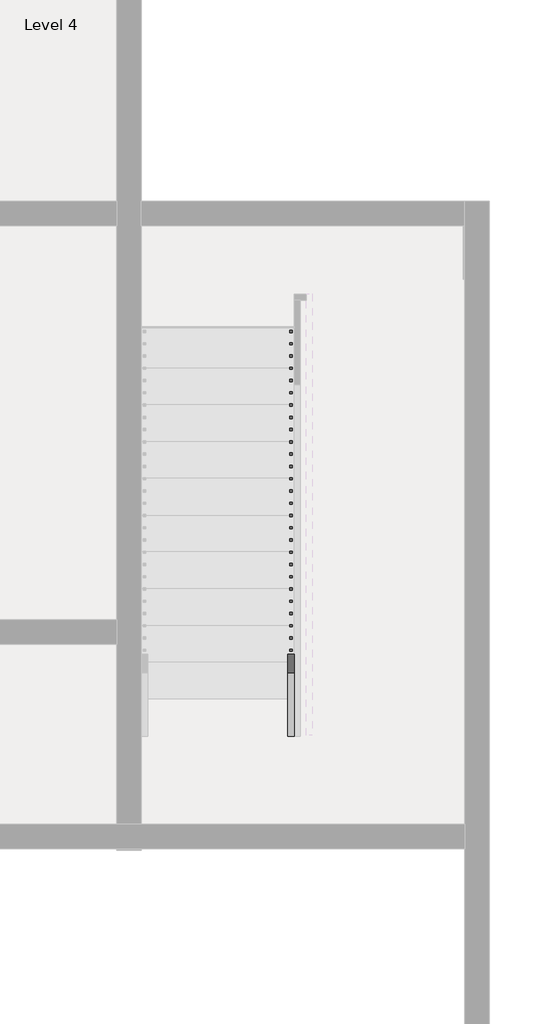
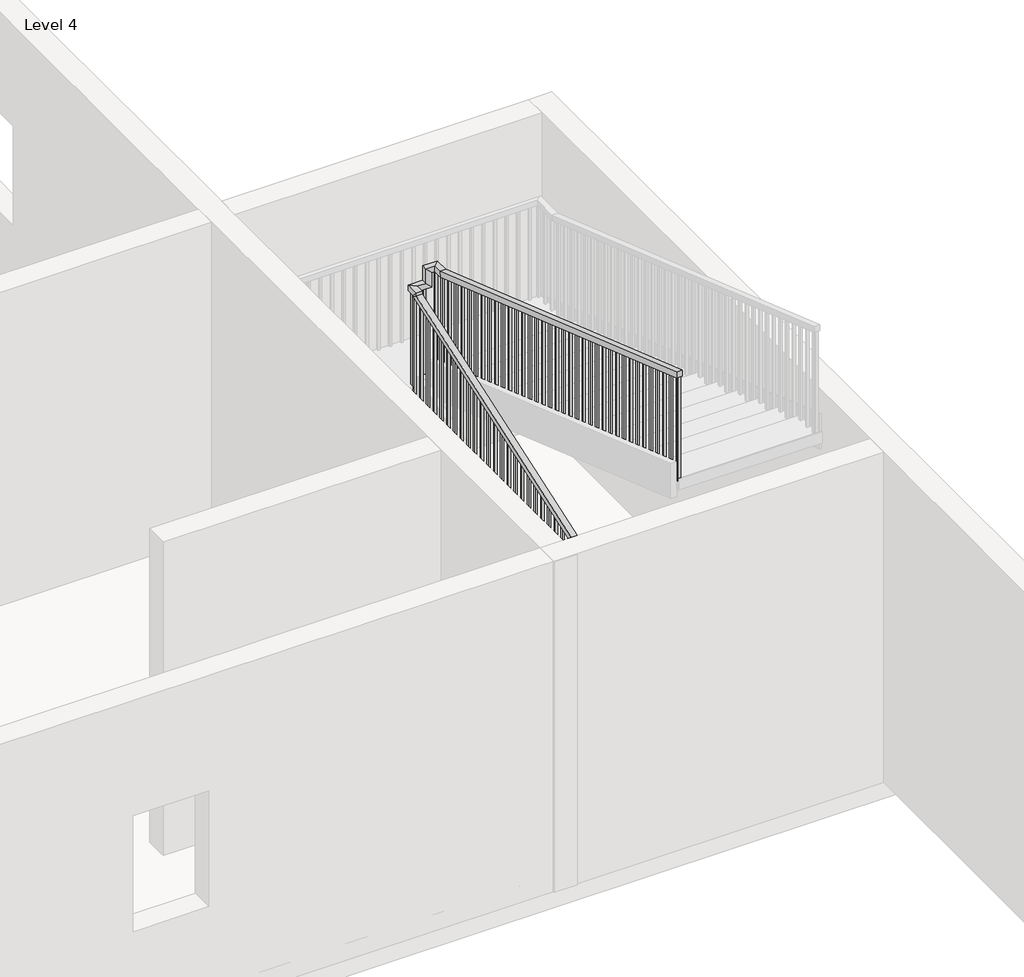
# One storey, part 6 of 14: 1 railing.
"""IFC4 building model written with IfcOpenShell, lengths in millimetres."""

from ifc_helpers import new_model, si_unit, frame, origin, place, context, project, spatial, polyline, outline, extrude, faceted_brep, element, save

model = new_model("IFC4")

# Units and contexts
model_context = context("Model", 3, world=origin())
ifc_project = project(units=[si_unit("LENGTHUNIT", "METRE", prefix="MILLI")], contexts=[model_context])

# Site, building, storey
site = spatial("IfcSite", under=ifc_project)
building = spatial("IfcBuilding", under=site)
storey = spatial("IfcBuildingStorey", under=building, Name="Level 4", Elevation=9144.0)

# Railing
placement = place(None, origin())
element("IfcRailing", 1, ObjectType="Handrail - Rectangular", at=placement, inside=storey, context=model_context, shape_type="SolidModel", body=[
    faceted_brep([(-2644.5381751, -9955.5916506, 10163.9076923), (-2644.5381751, -9955.5916506, 10110.1602476), (-2593.7381751, -9955.5916506, 10110.1602476), (-2593.7381751, -9955.5916506, 10163.9076923), (-2644.5381751, -6367.8416506, 11403.6687908), (-2644.5381751, -6317.0416506, 11367.4754856), (-2593.7381751, -6317.0416506, 11367.4754856), (-2593.7381751, -6367.8416506, 11403.6687908), (-2644.5381751, -6367.8416506, 11430.0), (-2644.5381751, -6317.0416506, 11379.2), (-2593.7381751, -6317.0416506, 11379.2), (-2593.7381751, -6367.8416506, 11430.0), (-2644.5381751, -6240.8416506, 11430.0), (-2644.5381751, -6240.8416506, 11379.2), (-2593.7381751, -6291.6416506, 11379.2), (-2593.7381751, -6291.6416506, 11430.0), (-2517.5381751, -6240.8416506, 11430.0), (-2466.7381751, -6240.8416506, 11379.2), (-2466.7381751, -6291.6416506, 11379.2), (-2517.5381751, -6291.6416506, 11430.0), (-2517.5381751, -6240.8416506, 11561.8846154), (-2466.7381751, -6240.8416506, 11511.0846154), (-2466.7381751, -6291.6416506, 11511.0846154), (-2517.5381751, -6291.6416506, 11561.8846154), (-2390.5381751, -6240.8416506, 11561.8846154), (-2390.5381751, -6240.8416506, 11511.0846154), (-2441.3381751, -6291.6416506, 11511.0846154), (-2441.3381751, -6291.6416506, 11561.8846154), (-2390.5381751, -6367.8416506, 11561.8846154), (-2390.5381751, -6376.3852679, 11511.0846154), (-2441.3381751, -6376.3852679, 11511.0846154), (-2441.3381751, -6367.8416506, 11561.8846154), (-2390.5381751, -9949.2416506, 12801.6), (-2441.3381751, -9949.2416506, 12801.6), (-2441.3381751, -9949.2416506, 12747.842594), (-2390.5381751, -9949.2416506, 12747.842594)], [[[0, 1, 2, 3]], [[1, 0, 4, 5]], [[2, 1, 5, 6]], [[3, 2, 6, 7]], [[0, 3, 7, 4]], [[5, 4, 8, 9]], [[6, 5, 9, 10]], [[7, 6, 10, 11]], [[4, 7, 11, 8]], [[9, 8, 12, 13]], [[10, 9, 13, 14]], [[11, 10, 14, 15]], [[8, 11, 15, 12]], [[13, 12, 16, 17]], [[14, 13, 17, 18]], [[15, 14, 18, 19]], [[12, 15, 19, 16]], [[17, 16, 20, 21]], [[18, 17, 21, 22]], [[19, 18, 22, 23]], [[16, 19, 23, 20]], [[21, 20, 24, 25]], [[22, 21, 25, 26]], [[23, 22, 26, 27]], [[20, 23, 27, 24]], [[25, 24, 28, 29]], [[26, 25, 29, 30]], [[27, 26, 30, 31]], [[24, 27, 31, 28]], [[32, 33, 34, 35]], [[29, 28, 32, 35]], [[30, 29, 35, 34]], [[31, 30, 34, 33]], [[28, 31, 33, 32]]]),
    extrude(outline(polyline([(-9933.3666506, 12742.3474017), (-9914.3166506, 12735.7531709), (-9914.3166506, 11781.6923077), (-9933.3666506, 11781.6923077), (-9933.3666506, 12742.3474017)])), frame((-2425.4631751, 0.0, 0.0), z_axis=(1.0, 0.0, 0.0), x_axis=(0.0, 1.0, 0.0)), (0.0, 0.0, 1.0), 19.05),
    extrude(outline(polyline([(-9831.7666506, 12707.1781709), (-9812.7166506, 12700.5839402), (-9812.7166506, 11781.6923077), (-9831.7666506, 11781.6923077), (-9831.7666506, 12707.1781709)])), frame((-2425.4631751, 0.0, 0.0), z_axis=(1.0, 0.0, 0.0), x_axis=(0.0, 1.0, 0.0)), (0.0, 0.0, 1.0), 19.05),
    extrude(outline(polyline([(-9730.1666506, 12672.0089402), (-9711.1166506, 12665.4147094), (-9711.1166506, 11781.6923077), (-9730.1666506, 11781.6923077), (-9730.1666506, 12672.0089402)])), frame((-2425.4631751, 0.0, 0.0), z_axis=(1.0, 0.0, 0.0), x_axis=(0.0, 1.0, 0.0)), (0.0, 0.0, 1.0), 19.05),
    extrude(outline(polyline([(-9628.5666506, 12636.8397094), (-9609.5166506, 12630.2454786), (-9609.5166506, 11676.1846154), (-9628.5666506, 11676.1846154), (-9628.5666506, 12636.8397094)])), frame((-2425.4631751, 0.0, 0.0), z_axis=(1.0, 0.0, 0.0), x_axis=(0.0, 1.0, 0.0)), (0.0, 0.0, 1.0), 19.05),
    extrude(outline(polyline([(-9526.9666506, 12601.6704786), (-9507.9166506, 12595.0762479), (-9507.9166506, 11676.1846154), (-9526.9666506, 11676.1846154), (-9526.9666506, 12601.6704786)])), frame((-2425.4631751, 0.0, 0.0), z_axis=(1.0, 0.0, 0.0), x_axis=(0.0, 1.0, 0.0)), (0.0, 0.0, 1.0), 19.05),
    extrude(outline(polyline([(-9425.3666506, 12566.5012479), (-9406.3166506, 12559.9070171), (-9406.3166506, 11676.1846154), (-9425.3666506, 11676.1846154), (-9425.3666506, 12566.5012479)])), frame((-2425.4631751, 0.0, 0.0), z_axis=(1.0, 0.0, 0.0), x_axis=(0.0, 1.0, 0.0)), (0.0, 0.0, 1.0), 19.05),
    extrude(outline(polyline([(-9323.7666506, 12531.3320171), (-9304.7166506, 12524.7377863), (-9304.7166506, 11570.6769231), (-9323.7666506, 11570.6769231), (-9323.7666506, 12531.3320171)])), frame((-2425.4631751, 0.0, 0.0), z_axis=(1.0, 0.0, 0.0), x_axis=(0.0, 1.0, 0.0)), (0.0, 0.0, 1.0), 19.05),
    extrude(outline(polyline([(-9222.1666506, 12496.1627863), (-9203.1166506, 12489.5685556), (-9203.1166506, 11570.6769231), (-9222.1666506, 11570.6769231), (-9222.1666506, 12496.1627863)])), frame((-2425.4631751, 0.0, 0.0), z_axis=(1.0, 0.0, 0.0), x_axis=(0.0, 1.0, 0.0)), (0.0, 0.0, 1.0), 19.05),
    extrude(outline(polyline([(-9120.5666506, 12460.9935556), (-9101.5166506, 12454.3993248), (-9101.5166506, 11570.6769231), (-9120.5666506, 11570.6769231), (-9120.5666506, 12460.9935556)])), frame((-2425.4631751, 0.0, 0.0), z_axis=(1.0, 0.0, 0.0), x_axis=(0.0, 1.0, 0.0)), (0.0, 0.0, 1.0), 19.05),
    extrude(outline(polyline([(-9018.9666506, 12425.8243248), (-8999.9166506, 12419.230094), (-8999.9166506, 11465.1692308), (-9018.9666506, 11465.1692308), (-9018.9666506, 12425.8243248)])), frame((-2425.4631751, 0.0, 0.0), z_axis=(1.0, 0.0, 0.0), x_axis=(0.0, 1.0, 0.0)), (0.0, 0.0, 1.0), 19.05),
    extrude(outline(polyline([(-8917.3666506, 12390.655094), (-8898.3166506, 12384.0608632), (-8898.3166506, 11465.1692308), (-8917.3666506, 11465.1692308), (-8917.3666506, 12390.655094)])), frame((-2425.4631751, 0.0, 0.0), z_axis=(1.0, 0.0, 0.0), x_axis=(0.0, 1.0, 0.0)), (0.0, 0.0, 1.0), 19.05),
    extrude(outline(polyline([(-8815.7666506, 12355.4858632), (-8796.7166506, 12348.8916325), (-8796.7166506, 11465.1692308), (-8815.7666506, 11465.1692308), (-8815.7666506, 12355.4858632)])), frame((-2425.4631751, 0.0, 0.0), z_axis=(1.0, 0.0, 0.0), x_axis=(0.0, 1.0, 0.0)), (0.0, 0.0, 1.0), 19.05),
    extrude(outline(polyline([(-8714.1666506, 12320.3166325), (-8695.1166506, 12313.7224017), (-8695.1166506, 11359.6615385), (-8714.1666506, 11359.6615385), (-8714.1666506, 12320.3166325)])), frame((-2425.4631751, 0.0, 0.0), z_axis=(1.0, 0.0, 0.0), x_axis=(0.0, 1.0, 0.0)), (0.0, 0.0, 1.0), 19.05),
    extrude(outline(polyline([(-8612.5666506, 12285.1474017), (-8593.5166506, 12278.5531709), (-8593.5166506, 11359.6615385), (-8612.5666506, 11359.6615385), (-8612.5666506, 12285.1474017)])), frame((-2425.4631751, 0.0, 0.0), z_axis=(1.0, 0.0, 0.0), x_axis=(0.0, 1.0, 0.0)), (0.0, 0.0, 1.0), 19.05),
    extrude(outline(polyline([(-8510.9666506, 12249.9781709), (-8491.9166506, 12243.3839402), (-8491.9166506, 11359.6615385), (-8510.9666506, 11359.6615385), (-8510.9666506, 12249.9781709)])), frame((-2425.4631751, 0.0, 0.0), z_axis=(1.0, 0.0, 0.0), x_axis=(0.0, 1.0, 0.0)), (0.0, 0.0, 1.0), 19.05),
    extrude(outline(polyline([(-8409.3666506, 12214.8089402), (-8390.3166506, 12208.2147094), (-8390.3166506, 11254.1538462), (-8409.3666506, 11254.1538462), (-8409.3666506, 12214.8089402)])), frame((-2425.4631751, 0.0, 0.0), z_axis=(1.0, 0.0, 0.0), x_axis=(0.0, 1.0, 0.0)), (0.0, 0.0, 1.0), 19.05),
    extrude(outline(polyline([(-8307.7666506, 12179.6397094), (-8288.7166506, 12173.0454786), (-8288.7166506, 11254.1538462), (-8307.7666506, 11254.1538462), (-8307.7666506, 12179.6397094)])), frame((-2425.4631751, 0.0, 0.0), z_axis=(1.0, 0.0, 0.0), x_axis=(0.0, 1.0, 0.0)), (0.0, 0.0, 1.0), 19.05),
    extrude(outline(polyline([(-8206.1666506, 12144.4704786), (-8187.1166506, 12137.8762479), (-8187.1166506, 11254.1538462), (-8206.1666506, 11254.1538462), (-8206.1666506, 12144.4704786)])), frame((-2425.4631751, 0.0, 0.0), z_axis=(1.0, 0.0, 0.0), x_axis=(0.0, 1.0, 0.0)), (0.0, 0.0, 1.0), 19.05),
    extrude(outline(polyline([(-8104.5666506, 12109.3012479), (-8085.5166506, 12102.7070171), (-8085.5166506, 11148.6461538), (-8104.5666506, 11148.6461538), (-8104.5666506, 12109.3012479)])), frame((-2425.4631751, 0.0, 0.0), z_axis=(1.0, 0.0, 0.0), x_axis=(0.0, 1.0, 0.0)), (0.0, 0.0, 1.0), 19.05),
    extrude(outline(polyline([(-8002.9666506, 12074.1320171), (-7983.9166506, 12067.5377863), (-7983.9166506, 11148.6461538), (-8002.9666506, 11148.6461538), (-8002.9666506, 12074.1320171)])), frame((-2425.4631751, 0.0, 0.0), z_axis=(1.0, 0.0, 0.0), x_axis=(0.0, 1.0, 0.0)), (0.0, 0.0, 1.0), 19.05),
    extrude(outline(polyline([(-7901.3666506, 12038.9627863), (-7882.3166506, 12032.3685556), (-7882.3166506, 11148.6461538), (-7901.3666506, 11148.6461538), (-7901.3666506, 12038.9627863)])), frame((-2425.4631751, 0.0, 0.0), z_axis=(1.0, 0.0, 0.0), x_axis=(0.0, 1.0, 0.0)), (0.0, 0.0, 1.0), 19.05),
    extrude(outline(polyline([(-7799.7666506, 12003.7935556), (-7780.7166506, 11997.1993248), (-7780.7166506, 11043.1384615), (-7799.7666506, 11043.1384615), (-7799.7666506, 12003.7935556)])), frame((-2425.4631751, 0.0, 0.0), z_axis=(1.0, 0.0, 0.0), x_axis=(0.0, 1.0, 0.0)), (0.0, 0.0, 1.0), 19.05),
    extrude(outline(polyline([(-7698.1666506, 11968.6243248), (-7679.1166506, 11962.030094), (-7679.1166506, 11043.1384615), (-7698.1666506, 11043.1384615), (-7698.1666506, 11968.6243248)])), frame((-2425.4631751, 0.0, 0.0), z_axis=(1.0, 0.0, 0.0), x_axis=(0.0, 1.0, 0.0)), (0.0, 0.0, 1.0), 19.05),
    extrude(outline(polyline([(-7596.5666506, 11933.455094), (-7577.5166506, 11926.8608632), (-7577.5166506, 11043.1384615), (-7596.5666506, 11043.1384615), (-7596.5666506, 11933.455094)])), frame((-2425.4631751, 0.0, 0.0), z_axis=(1.0, 0.0, 0.0), x_axis=(0.0, 1.0, 0.0)), (0.0, 0.0, 1.0), 19.05),
    extrude(outline(polyline([(-7494.9666506, 11898.2858632), (-7475.9166506, 11891.6916325), (-7475.9166506, 10937.6307692), (-7494.9666506, 10937.6307692), (-7494.9666506, 11898.2858632)])), frame((-2425.4631751, 0.0, 0.0), z_axis=(1.0, 0.0, 0.0), x_axis=(0.0, 1.0, 0.0)), (0.0, 0.0, 1.0), 19.05),
    extrude(outline(polyline([(-7393.3666506, 11863.1166325), (-7374.3166506, 11856.5224017), (-7374.3166506, 10937.6307692), (-7393.3666506, 10937.6307692), (-7393.3666506, 11863.1166325)])), frame((-2425.4631751, 0.0, 0.0), z_axis=(1.0, 0.0, 0.0), x_axis=(0.0, 1.0, 0.0)), (0.0, 0.0, 1.0), 19.05),
    extrude(outline(polyline([(-7291.7666506, 11827.9474017), (-7272.7166506, 11821.3531709), (-7272.7166506, 10937.6307692), (-7291.7666506, 10937.6307692), (-7291.7666506, 11827.9474017)])), frame((-2425.4631751, 0.0, 0.0), z_axis=(1.0, 0.0, 0.0), x_axis=(0.0, 1.0, 0.0)), (0.0, 0.0, 1.0), 19.05),
    extrude(outline(polyline([(-7190.1666506, 11792.7781709), (-7171.1166506, 11786.1839402), (-7171.1166506, 10832.1230769), (-7190.1666506, 10832.1230769), (-7190.1666506, 11792.7781709)])), frame((-2425.4631751, 0.0, 0.0), z_axis=(1.0, 0.0, 0.0), x_axis=(0.0, 1.0, 0.0)), (0.0, 0.0, 1.0), 19.05),
    extrude(outline(polyline([(-7088.5666506, 11757.6089402), (-7069.5166506, 11751.0147094), (-7069.5166506, 10832.1230769), (-7088.5666506, 10832.1230769), (-7088.5666506, 11757.6089402)])), frame((-2425.4631751, 0.0, 0.0), z_axis=(1.0, 0.0, 0.0), x_axis=(0.0, 1.0, 0.0)), (0.0, 0.0, 1.0), 19.05),
    extrude(outline(polyline([(-6986.9666506, 11722.4397094), (-6967.9166506, 11715.8454786), (-6967.9166506, 10832.1230769), (-6986.9666506, 10832.1230769), (-6986.9666506, 11722.4397094)])), frame((-2425.4631751, 0.0, 0.0), z_axis=(1.0, 0.0, 0.0), x_axis=(0.0, 1.0, 0.0)), (0.0, 0.0, 1.0), 19.05),
    extrude(outline(polyline([(-6885.3666506, 11687.2704786), (-6866.3166506, 11680.6762479), (-6866.3166506, 10726.6153846), (-6885.3666506, 10726.6153846), (-6885.3666506, 11687.2704786)])), frame((-2425.4631751, 0.0, 0.0), z_axis=(1.0, 0.0, 0.0), x_axis=(0.0, 1.0, 0.0)), (0.0, 0.0, 1.0), 19.05),
    extrude(outline(polyline([(-6783.7666506, 11652.1012479), (-6764.7166506, 11645.5070171), (-6764.7166506, 10726.6153846), (-6783.7666506, 10726.6153846), (-6783.7666506, 11652.1012479)])), frame((-2425.4631751, 0.0, 0.0), z_axis=(1.0, 0.0, 0.0), x_axis=(0.0, 1.0, 0.0)), (0.0, 0.0, 1.0), 19.05),
    extrude(outline(polyline([(-6682.1666506, 11616.9320171), (-6663.1166506, 11610.3377863), (-6663.1166506, 10726.6153846), (-6682.1666506, 10726.6153846), (-6682.1666506, 11616.9320171)])), frame((-2425.4631751, 0.0, 0.0), z_axis=(1.0, 0.0, 0.0), x_axis=(0.0, 1.0, 0.0)), (0.0, 0.0, 1.0), 19.05),
    extrude(outline(polyline([(-6580.5666506, 11581.7627863), (-6561.5166506, 11575.1685556), (-6561.5166506, 10621.1076923), (-6580.5666506, 10621.1076923), (-6580.5666506, 11581.7627863)])), frame((-2425.4631751, 0.0, 0.0), z_axis=(1.0, 0.0, 0.0), x_axis=(0.0, 1.0, 0.0)), (0.0, 0.0, 1.0), 19.05),
    extrude(outline(polyline([(-6478.9666506, 11546.5935556), (-6459.9166506, 11539.9993248), (-6459.9166506, 10621.1076923), (-6478.9666506, 10621.1076923), (-6478.9666506, 11546.5935556)])), frame((-2425.4631751, 0.0, 0.0), z_axis=(1.0, 0.0, 0.0), x_axis=(0.0, 1.0, 0.0)), (0.0, 0.0, 1.0), 19.05),
    extrude(outline(polyline([(-6377.3666506, 11511.4243248), (-6358.3166506, 11504.830094), (-6358.3166506, 10621.1076923), (-6377.3666506, 10621.1076923), (-6377.3666506, 11511.4243248)])), frame((-2425.4631751, 0.0, 0.0), z_axis=(1.0, 0.0, 0.0), x_axis=(0.0, 1.0, 0.0)), (0.0, 0.0, 1.0), 19.05),
    extrude(outline(polyline([(-2527.0631751, -6275.7666506), (-2527.0631751, -6256.7166506), (-2508.0131751, -6256.7166506), (-2508.0131751, -6275.7666506), (-2527.0631751, -6275.7666506)])), frame((0.0, 0.0, 10515.6), z_axis=(0.0, 0.0, 1.0), x_axis=(1.0, 0.0, 0.0)), (0.0, 0.0, 1.0), 863.6),
    extrude(outline(polyline([(-2609.6131751, -6307.5166506), (-2628.6631751, -6307.5166506), (-2628.6631751, -6288.4666506), (-2609.6131751, -6288.4666506), (-2609.6131751, -6307.5166506)])), frame((0.0, 0.0, 10410.0923077), z_axis=(0.0, 0.0, 1.0), x_axis=(1.0, 0.0, 0.0)), (0.0, 0.0, 1.0), 969.1076923),
    extrude(outline(polyline([(-6409.1166506, 11335.6586078), (-6390.0666506, 11342.2414101), (-6390.0666506, 10410.0923077), (-6409.1166506, 10410.0923077), (-6409.1166506, 11335.6586078)])), frame((-2628.6631751, 0.0, 0.0), z_axis=(1.0, 0.0, 0.0), x_axis=(0.0, 1.0, 0.0)), (0.0, 0.0, 1.0), 19.05),
    extrude(outline(polyline([(-6510.7166506, 11300.5503289), (-6491.6666506, 11307.1331312), (-6491.6666506, 10410.0923077), (-6510.7166506, 10410.0923077), (-6510.7166506, 11300.5503289)])), frame((-2628.6631751, 0.0, 0.0), z_axis=(1.0, 0.0, 0.0), x_axis=(0.0, 1.0, 0.0)), (0.0, 0.0, 1.0), 19.05),
    extrude(outline(polyline([(-6612.3166506, 11265.44205), (-6593.2666506, 11272.0248523), (-6593.2666506, 10304.5846154), (-6612.3166506, 10304.5846154), (-6612.3166506, 11265.44205)])), frame((-2628.6631751, 0.0, 0.0), z_axis=(1.0, 0.0, 0.0), x_axis=(0.0, 1.0, 0.0)), (0.0, 0.0, 1.0), 19.05),
    extrude(outline(polyline([(-6713.9166506, 11230.3337711), (-6694.8666506, 11236.9165734), (-6694.8666506, 10304.5846154), (-6713.9166506, 10304.5846154), (-6713.9166506, 11230.3337711)])), frame((-2628.6631751, 0.0, 0.0), z_axis=(1.0, 0.0, 0.0), x_axis=(0.0, 1.0, 0.0)), (0.0, 0.0, 1.0), 19.05),
    extrude(outline(polyline([(-6815.5166506, 11195.2254922), (-6796.4666506, 11201.8082945), (-6796.4666506, 10304.5846154), (-6815.5166506, 10304.5846154), (-6815.5166506, 11195.2254922)])), frame((-2628.6631751, 0.0, 0.0), z_axis=(1.0, 0.0, 0.0), x_axis=(0.0, 1.0, 0.0)), (0.0, 0.0, 1.0), 19.05),
    extrude(outline(polyline([(-6917.1166506, 11160.1172133), (-6898.0666506, 11166.7000156), (-6898.0666506, 10199.0769231), (-6917.1166506, 10199.0769231), (-6917.1166506, 11160.1172133)])), frame((-2628.6631751, 0.0, 0.0), z_axis=(1.0, 0.0, 0.0), x_axis=(0.0, 1.0, 0.0)), (0.0, 0.0, 1.0), 19.05),
    extrude(outline(polyline([(-7018.7166506, 11125.0089344), (-6999.6666506, 11131.5917367), (-6999.6666506, 10199.0769231), (-7018.7166506, 10199.0769231), (-7018.7166506, 11125.0089344)])), frame((-2628.6631751, 0.0, 0.0), z_axis=(1.0, 0.0, 0.0), x_axis=(0.0, 1.0, 0.0)), (0.0, 0.0, 1.0), 19.05),
    extrude(outline(polyline([(-7120.3166506, 11089.9006556), (-7101.2666506, 11096.4834578), (-7101.2666506, 10199.0769231), (-7120.3166506, 10199.0769231), (-7120.3166506, 11089.9006556)])), frame((-2628.6631751, 0.0, 0.0), z_axis=(1.0, 0.0, 0.0), x_axis=(0.0, 1.0, 0.0)), (0.0, 0.0, 1.0), 19.05),
    extrude(outline(polyline([(-7221.9166506, 11054.7923767), (-7202.8666506, 11061.375179), (-7202.8666506, 10093.5692308), (-7221.9166506, 10093.5692308), (-7221.9166506, 11054.7923767)])), frame((-2628.6631751, 0.0, 0.0), z_axis=(1.0, 0.0, 0.0), x_axis=(0.0, 1.0, 0.0)), (0.0, 0.0, 1.0), 19.05),
    extrude(outline(polyline([(-7323.5166506, 11019.6840978), (-7304.4666506, 11026.2669001), (-7304.4666506, 10093.5692308), (-7323.5166506, 10093.5692308), (-7323.5166506, 11019.6840978)])), frame((-2628.6631751, 0.0, 0.0), z_axis=(1.0, 0.0, 0.0), x_axis=(0.0, 1.0, 0.0)), (0.0, 0.0, 1.0), 19.05),
    extrude(outline(polyline([(-7425.1166506, 10984.5758189), (-7406.0666506, 10991.1586212), (-7406.0666506, 10093.5692308), (-7425.1166506, 10093.5692308), (-7425.1166506, 10984.5758189)])), frame((-2628.6631751, 0.0, 0.0), z_axis=(1.0, 0.0, 0.0), x_axis=(0.0, 1.0, 0.0)), (0.0, 0.0, 1.0), 19.05),
    extrude(outline(polyline([(-7526.7166506, 10949.46754), (-7507.6666506, 10956.0503423), (-7507.6666506, 9988.0615385), (-7526.7166506, 9988.0615385), (-7526.7166506, 10949.46754)])), frame((-2628.6631751, 0.0, 0.0), z_axis=(1.0, 0.0, 0.0), x_axis=(0.0, 1.0, 0.0)), (0.0, 0.0, 1.0), 19.05),
    extrude(outline(polyline([(-7628.3166506, 10914.3592611), (-7609.2666506, 10920.9420634), (-7609.2666506, 9988.0615385), (-7628.3166506, 9988.0615385), (-7628.3166506, 10914.3592611)])), frame((-2628.6631751, 0.0, 0.0), z_axis=(1.0, 0.0, 0.0), x_axis=(0.0, 1.0, 0.0)), (0.0, 0.0, 1.0), 19.05),
    extrude(outline(polyline([(-7729.9166506, 10879.2509822), (-7710.8666506, 10885.8337845), (-7710.8666506, 9988.0615385), (-7729.9166506, 9988.0615385), (-7729.9166506, 10879.2509822)])), frame((-2628.6631751, 0.0, 0.0), z_axis=(1.0, 0.0, 0.0), x_axis=(0.0, 1.0, 0.0)), (0.0, 0.0, 1.0), 19.05),
    extrude(outline(polyline([(-7831.5166506, 10844.1427033), (-7812.4666506, 10850.7255056), (-7812.4666506, 9882.5538462), (-7831.5166506, 9882.5538462), (-7831.5166506, 10844.1427033)])), frame((-2628.6631751, 0.0, 0.0), z_axis=(1.0, 0.0, 0.0), x_axis=(0.0, 1.0, 0.0)), (0.0, 0.0, 1.0), 19.05),
    extrude(outline(polyline([(-7933.1166506, 10809.0344244), (-7914.0666506, 10815.6172267), (-7914.0666506, 9882.5538462), (-7933.1166506, 9882.5538462), (-7933.1166506, 10809.0344244)])), frame((-2628.6631751, 0.0, 0.0), z_axis=(1.0, 0.0, 0.0), x_axis=(0.0, 1.0, 0.0)), (0.0, 0.0, 1.0), 19.05),
    extrude(outline(polyline([(-8034.7166506, 10773.9261455), (-8015.6666506, 10780.5089478), (-8015.6666506, 9882.5538462), (-8034.7166506, 9882.5538462), (-8034.7166506, 10773.9261455)])), frame((-2628.6631751, 0.0, 0.0), z_axis=(1.0, 0.0, 0.0), x_axis=(0.0, 1.0, 0.0)), (0.0, 0.0, 1.0), 19.05),
    extrude(outline(polyline([(-8136.3166506, 10738.8178666), (-8117.2666506, 10745.4006689), (-8117.2666506, 9777.0461538), (-8136.3166506, 9777.0461538), (-8136.3166506, 10738.8178666)])), frame((-2628.6631751, 0.0, 0.0), z_axis=(1.0, 0.0, 0.0), x_axis=(0.0, 1.0, 0.0)), (0.0, 0.0, 1.0), 19.05),
    extrude(outline(polyline([(-8237.9166506, 10703.7095877), (-8218.8666506, 10710.29239), (-8218.8666506, 9777.0461538), (-8237.9166506, 9777.0461538), (-8237.9166506, 10703.7095877)])), frame((-2628.6631751, 0.0, 0.0), z_axis=(1.0, 0.0, 0.0), x_axis=(0.0, 1.0, 0.0)), (0.0, 0.0, 1.0), 19.05),
    extrude(outline(polyline([(-8339.5166506, 10668.6013088), (-8320.4666506, 10675.1841111), (-8320.4666506, 9777.0461538), (-8339.5166506, 9777.0461538), (-8339.5166506, 10668.6013088)])), frame((-2628.6631751, 0.0, 0.0), z_axis=(1.0, 0.0, 0.0), x_axis=(0.0, 1.0, 0.0)), (0.0, 0.0, 1.0), 19.05),
    extrude(outline(polyline([(-8441.1166506, 10633.4930299), (-8422.0666506, 10640.0758322), (-8422.0666506, 9671.5384615), (-8441.1166506, 9671.5384615), (-8441.1166506, 10633.4930299)])), frame((-2628.6631751, 0.0, 0.0), z_axis=(1.0, 0.0, 0.0), x_axis=(0.0, 1.0, 0.0)), (0.0, 0.0, 1.0), 19.05),
    extrude(outline(polyline([(-8542.7166506, 10598.384751), (-8523.6666506, 10604.9675533), (-8523.6666506, 9671.5384615), (-8542.7166506, 9671.5384615), (-8542.7166506, 10598.384751)])), frame((-2628.6631751, 0.0, 0.0), z_axis=(1.0, 0.0, 0.0), x_axis=(0.0, 1.0, 0.0)), (0.0, 0.0, 1.0), 19.05),
    extrude(outline(polyline([(-8644.3166506, 10563.2764721), (-8625.2666506, 10569.8592744), (-8625.2666506, 9671.5384615), (-8644.3166506, 9671.5384615), (-8644.3166506, 10563.2764721)])), frame((-2628.6631751, 0.0, 0.0), z_axis=(1.0, 0.0, 0.0), x_axis=(0.0, 1.0, 0.0)), (0.0, 0.0, 1.0), 19.05),
    extrude(outline(polyline([(-8745.9166506, 10528.1681932), (-8726.8666506, 10534.7509955), (-8726.8666506, 9566.0307692), (-8745.9166506, 9566.0307692), (-8745.9166506, 10528.1681932)])), frame((-2628.6631751, 0.0, 0.0), z_axis=(1.0, 0.0, 0.0), x_axis=(0.0, 1.0, 0.0)), (0.0, 0.0, 1.0), 19.05),
    extrude(outline(polyline([(-8847.5166506, 10493.0599143), (-8828.4666506, 10499.6427166), (-8828.4666506, 9566.0307692), (-8847.5166506, 9566.0307692), (-8847.5166506, 10493.0599143)])), frame((-2628.6631751, 0.0, 0.0), z_axis=(1.0, 0.0, 0.0), x_axis=(0.0, 1.0, 0.0)), (0.0, 0.0, 1.0), 19.05),
    extrude(outline(polyline([(-8949.1166506, 10457.9516354), (-8930.0666506, 10464.5344377), (-8930.0666506, 9566.0307692), (-8949.1166506, 9566.0307692), (-8949.1166506, 10457.9516354)])), frame((-2628.6631751, 0.0, 0.0), z_axis=(1.0, 0.0, 0.0), x_axis=(0.0, 1.0, 0.0)), (0.0, 0.0, 1.0), 19.05),
    extrude(outline(polyline([(-9050.7166506, 10422.8433565), (-9031.6666506, 10429.4261588), (-9031.6666506, 9460.5230769), (-9050.7166506, 9460.5230769), (-9050.7166506, 10422.8433565)])), frame((-2628.6631751, 0.0, 0.0), z_axis=(1.0, 0.0, 0.0), x_axis=(0.0, 1.0, 0.0)), (0.0, 0.0, 1.0), 19.05),
    extrude(outline(polyline([(-9152.3166506, 10387.7350776), (-9133.2666506, 10394.3178799), (-9133.2666506, 9460.5230769), (-9152.3166506, 9460.5230769), (-9152.3166506, 10387.7350776)])), frame((-2628.6631751, 0.0, 0.0), z_axis=(1.0, 0.0, 0.0), x_axis=(0.0, 1.0, 0.0)), (0.0, 0.0, 1.0), 19.05),
    extrude(outline(polyline([(-9253.9166506, 10352.6267987), (-9234.8666506, 10359.209601), (-9234.8666506, 9460.5230769), (-9253.9166506, 9460.5230769), (-9253.9166506, 10352.6267987)])), frame((-2628.6631751, 0.0, 0.0), z_axis=(1.0, 0.0, 0.0), x_axis=(0.0, 1.0, 0.0)), (0.0, 0.0, 1.0), 19.05),
    extrude(outline(polyline([(-9355.5166506, 10317.5185198), (-9336.4666506, 10324.1013221), (-9336.4666506, 9355.0153846), (-9355.5166506, 9355.0153846), (-9355.5166506, 10317.5185198)])), frame((-2628.6631751, 0.0, 0.0), z_axis=(1.0, 0.0, 0.0), x_axis=(0.0, 1.0, 0.0)), (0.0, 0.0, 1.0), 19.05),
    extrude(outline(polyline([(-9457.1166506, 10282.4102409), (-9438.0666506, 10288.9930432), (-9438.0666506, 9355.0153846), (-9457.1166506, 9355.0153846), (-9457.1166506, 10282.4102409)])), frame((-2628.6631751, 0.0, 0.0), z_axis=(1.0, 0.0, 0.0), x_axis=(0.0, 1.0, 0.0)), (0.0, 0.0, 1.0), 19.05),
    extrude(outline(polyline([(-9558.7166506, 10247.301962), (-9539.6666506, 10253.8847643), (-9539.6666506, 9355.0153846), (-9558.7166506, 9355.0153846), (-9558.7166506, 10247.301962)])), frame((-2628.6631751, 0.0, 0.0), z_axis=(1.0, 0.0, 0.0), x_axis=(0.0, 1.0, 0.0)), (0.0, 0.0, 1.0), 19.05),
    extrude(outline(polyline([(-9660.3166506, 10212.1936831), (-9641.2666506, 10218.7764854), (-9641.2666506, 9249.5076923), (-9660.3166506, 9249.5076923), (-9660.3166506, 10212.1936831)])), frame((-2628.6631751, 0.0, 0.0), z_axis=(1.0, 0.0, 0.0), x_axis=(0.0, 1.0, 0.0)), (0.0, 0.0, 1.0), 19.05),
    extrude(outline(polyline([(-9761.9166506, 10177.0854043), (-9742.8666506, 10183.6682065), (-9742.8666506, 9249.5076923), (-9761.9166506, 9249.5076923), (-9761.9166506, 10177.0854043)])), frame((-2628.6631751, 0.0, 0.0), z_axis=(1.0, 0.0, 0.0), x_axis=(0.0, 1.0, 0.0)), (0.0, 0.0, 1.0), 19.05),
    extrude(outline(polyline([(-9863.5166506, 10141.9771254), (-9844.4666506, 10148.5599277), (-9844.4666506, 9249.5076923), (-9863.5166506, 9249.5076923), (-9863.5166506, 10141.9771254)])), frame((-2628.6631751, 0.0, 0.0), z_axis=(1.0, 0.0, 0.0), x_axis=(0.0, 1.0, 0.0)), (0.0, 0.0, 1.0), 19.05),
    extrude(outline(polyline([(-2425.4631751, -6275.7666506), (-2425.4631751, -6256.7166506), (-2406.4131751, -6256.7166506), (-2406.4131751, -6275.7666506), (-2425.4631751, -6275.7666506)])), frame((0.0, 0.0, 10515.6), z_axis=(0.0, 0.0, 1.0), x_axis=(1.0, 0.0, 0.0)), (0.0, 0.0, 1.0), 995.4846154),
    extrude(outline(polyline([(-2609.6131751, -6275.7666506), (-2628.6631751, -6275.7666506), (-2628.6631751, -6256.7166506), (-2609.6131751, -6256.7166506), (-2609.6131751, -6275.7666506)])), frame((0.0, 0.0, 10515.6), z_axis=(0.0, 0.0, 1.0), x_axis=(1.0, 0.0, 0.0)), (0.0, 0.0, 1.0), 863.6),
    extrude(outline(polyline([(-9949.2416506, 12747.842594), (-9930.1916506, 12741.2483632), (-9930.1916506, 11781.6923077), (-9949.2416506, 11781.6923077), (-9949.2416506, 12747.842594)])), frame((-2425.4631751, 0.0, 0.0), z_axis=(1.0, 0.0, 0.0), x_axis=(0.0, 1.0, 0.0)), (0.0, 0.0, 1.0), 19.05),
    extrude(outline(polyline([(-9955.5916506, 10110.1602476), (-9936.5416506, 10116.7430499), (-9936.5416506, 9249.5076923), (-9955.5916506, 9249.5076923), (-9955.5916506, 10110.1602476)])), frame((-2628.6631751, 0.0, 0.0), z_axis=(1.0, 0.0, 0.0), x_axis=(0.0, 1.0, 0.0)), (0.0, 0.0, 1.0), 19.05),
])

save(model, "model.ifc")

# Revit data of these elements
# Type "Handrail - Rectangular"
#   Assembly Code = "C2010400"
#   built-in parameter 1008612 = 0.0416667 (stored number, unit not read)
#   built-in parameter 1008611 = 0.0416667 (stored number, unit not read)
#   built-in parameter 1008609 = 0.333333 (stored number, unit not read)
#   built-in parameter 1008604 = 0.166667 (stored number, unit not read)
#   built-in parameter 1008603 = 0.166667 (stored number, unit not read)
#   Railing Height = 3' - 0"
#   built-in parameter 1008630 = 2
#   built-in parameter 1008610 = 2
#   built-in parameter 1008618 = Baluster - Square : 3/4"
# Element 1 (IfcRailing, "Handrail - Rectangular")
#   Phase Created = New Construction
